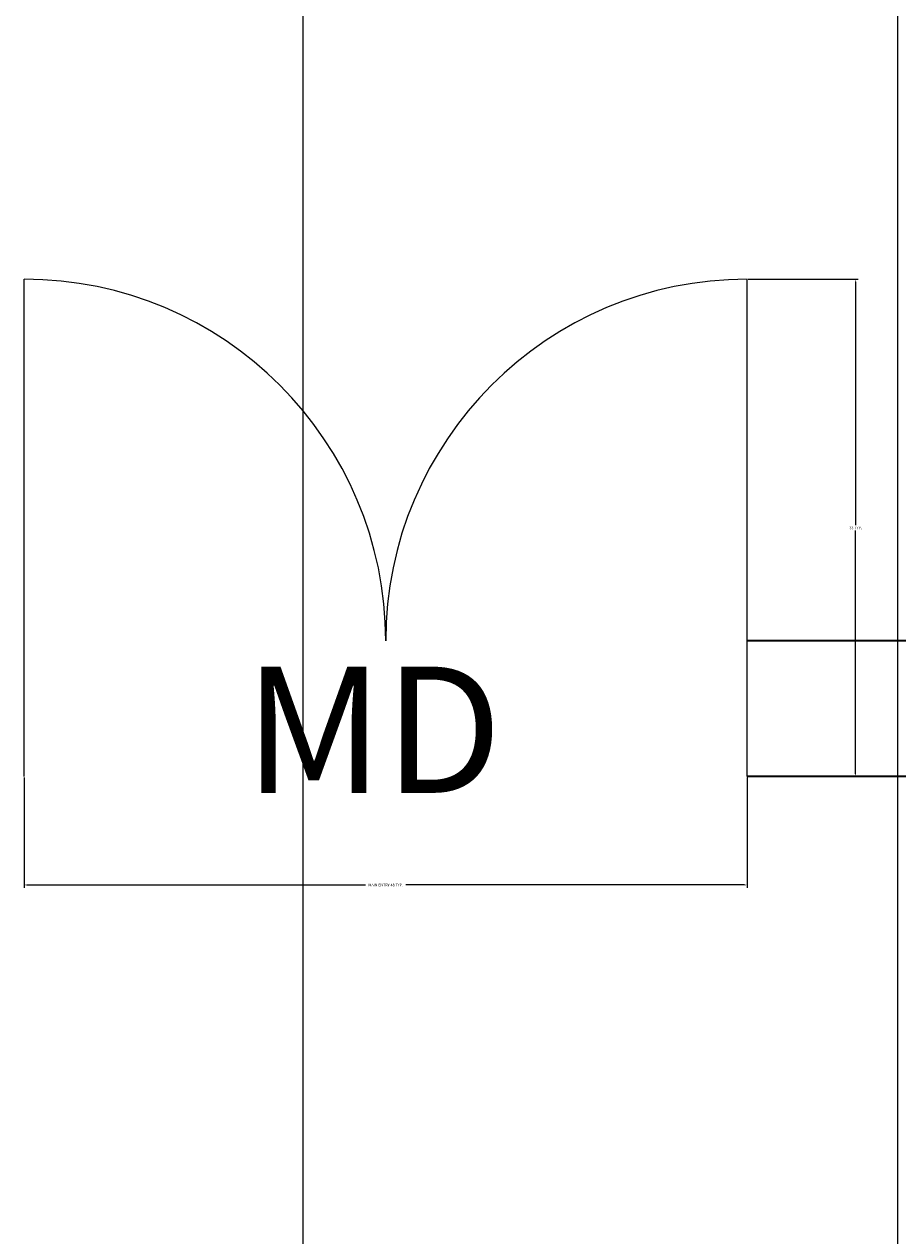
# Model space of a CAD drawing. Units: feet. Extents: x 1654 to 2985, y 1348 to 2230.
# Tile 44 of 53: x 2655 to 2713, y 1712 to 1792. Entities that reach past the tile are written whole.
import ezdxf

# ---------------------------------------------------------------- set-up
doc = ezdxf.new("R2010")
doc.units = ezdxf.units.FT
for name, color, linetype, lineweight in [('A-ANNO-DIMS', 2, 'Continuous', 18), ('A-ANNO-TEXT', 7, 'Continuous', 18), ('A-DOOR', 3, 'Continuous', 18), ('A-WALL', 7, 'Continuous', 35)]:
    doc.layers.add(name, color=color, linetype=linetype, lineweight=lineweight)
doc.styles.get("Standard").update_dxf_attribs({"font": 'arial.ttf'})
doc.dimstyles.get("Standard").update_dxf_attribs({"dimtxt": 0.18, "dimasz": 0.18, "dimexe": 0.18, "dimexo": 0.0625, "dimgap": 0.09, "dimtad": 0, "dimtih": 1, "dimtoh": 1, "dimdec": 4, "dimzin": 0, "dimdsep": 46, "dimtxsty": 'Standard', "dimcen": 0.09, "dimadec": 0, "dimazin": 0, "dimtfac": 1, "dimtdec": 4, "dimtofl": 0, "dimtmove": 0, "dimatfit": 3, "dimfxl": 1, "dimtolj": 1, "dimtzin": 0, "dimarcsym": 0})

# ---------------------------------------------------------------- blocks, each defined once
blk = doc.blocks.new('DOOR-ENTRY-PAIR')
for p, q in [((0, -9), (0, 24)), ((48, -9), (48, 24))]:
    blk.add_line(p, q)
for centre, start, end in [((0, 0), 0, 90), ((48, 0), 90, 180)]:
    blk.add_arc(centre, 24, start, end)
blk = doc.blocks.new('*D32')
at = {"layer": 'A-ANNO-DIMS', "color": 0, "lineweight": -2, "transparency": 16777216}
for p, q in [((2654.706, 1742.192), (2654.706, 1734.875)), ((2702.706, 1742.192), (2702.706, 1734.875)), ((2654.886, 1735.055), (2677.372, 1735.055)), ((2702.526, 1735.055), (2680.04, 1735.055))]:
    blk.add_line(p, q, dxfattribs=at)
at = {"layer": 'A-ANNO-DIMS', "color": 0, "transparency": 16777216}
for points in [[(2654.886, 1735.085), (2654.886, 1735.025), (2654.706, 1735.055)], [(2702.526, 1735.085), (2702.526, 1735.025), (2702.706, 1735.055)]]:
    blk.add_solid(points, dxfattribs=at)
at = {"layer": 'Defpoints', "color": 0, "transparency": 16777216}
for p in [(2654.706, 1742.255), (2702.706, 1742.255), (2702.706, 1735.055)]:
    blk.add_point(p, dxfattribs=at)
at = {"layer": 'A-ANNO-DIMS', "color": 0, "transparency": 16777216, "insert": (2678.706, 1735.055), "char_height": 0.18, "attachment_point": 5}
blk.add_mtext('\\A1;MAIN ENTRY 48 TYP.', dxfattribs=at)
blk = doc.blocks.new('*D33')
at = {"layer": 'A-ANNO-DIMS', "color": 0, "lineweight": -2, "transparency": 16777216}
for p, q in [((2702.768, 1775.255), (2710.086, 1775.255)), ((2709.906, 1775.075), (2709.906, 1758.937)), ((2709.906, 1742.435), (2709.906, 1758.573)), ((2702.768, 1742.255), (2710.086, 1742.255))]:
    blk.add_line(p, q, dxfattribs=at)
at = {"layer": 'A-ANNO-DIMS', "color": 0, "transparency": 16777216}
for points in [[(2709.876, 1775.075), (2709.936, 1775.075), (2709.906, 1775.255)], [(2709.876, 1742.435), (2709.936, 1742.435), (2709.906, 1742.255)]]:
    blk.add_solid(points, dxfattribs=at)
at = {"layer": 'Defpoints', "color": 0, "transparency": 16777216}
for p in [(2702.706, 1775.255), (2709.906, 1775.255), (2702.706, 1742.255)]:
    blk.add_point(p, dxfattribs=at)
at = {"layer": 'A-ANNO-DIMS', "color": 0, "transparency": 16777216, "insert": (2709.906, 1758.755), "char_height": 0.18, "attachment_point": 5}
blk.add_mtext('\\A1;33 TYP.', dxfattribs=at)
blk = doc.blocks.new('*D82')
at = {"layer": 'A-ANNO-DIMS', "color": 0, "lineweight": -2, "transparency": 16777216}
for p, q in [((2652.706, 2039.192), (2652.706, 1490.625)), ((2784.706, 2039.192), (2784.706, 1490.625)), ((2652.886, 1490.805), (2718.426, 1490.805)), ((2784.526, 1490.805), (2718.985, 1490.805))]:
    blk.add_line(p, q, dxfattribs=at)
at = {"layer": 'A-ANNO-DIMS', "color": 0, "transparency": 16777216}
for points in [[(2652.886, 1490.835), (2652.886, 1490.775), (2652.706, 1490.805)], [(2784.526, 1490.835), (2784.526, 1490.775), (2784.706, 1490.805)]]:
    blk.add_solid(points, dxfattribs=at)
at = {"layer": 'Defpoints', "color": 0, "transparency": 16777216}
for p in [(2652.706, 2039.255), (2784.706, 2039.255), (2784.706, 1490.805)]:
    blk.add_point(p, dxfattribs=at)
at = {"layer": 'A-ANNO-DIMS', "color": 0, "transparency": 16777216, "insert": (2718.706, 1490.805), "char_height": 0.18, "attachment_point": 5}
blk.add_mtext('\\A1;132', dxfattribs=at)
blk = doc.blocks.new('*D84')
at = {"layer": 'A-ANNO-DIMS', "color": 0, "lineweight": -2, "transparency": 16777216}
for p, q in [((2625.235, 1565.317), (2625.235, 2149.885)), ((2625.415, 2149.705), (2649.013, 2149.705)), ((2673.055, 2149.705), (2649.458, 2149.705)), ((2673.235, 1565.317), (2673.235, 2149.885))]:
    blk.add_line(p, q, dxfattribs=at)
at = {"layer": 'A-ANNO-DIMS', "color": 0, "transparency": 16777216}
for points in [[(2625.415, 2149.735), (2625.415, 2149.675), (2625.235, 2149.705)], [(2673.055, 2149.735), (2673.055, 2149.675), (2673.235, 2149.705)]]:
    blk.add_solid(points, dxfattribs=at)
at = {"layer": 'Defpoints', "color": 0, "transparency": 16777216}
for p in [(2673.235, 2149.705), (2625.235, 1565.255), (2673.235, 1565.255)]:
    blk.add_point(p, dxfattribs=at)
at = {"layer": 'A-ANNO-DIMS', "color": 0, "transparency": 16777216, "insert": (2649.235, 2149.705), "char_height": 0.18, "attachment_point": 5}
blk.add_mtext('\\A1;48', dxfattribs=at)
blk = doc.blocks.new('*D85')
at = {"layer": 'A-ANNO-DIMS', "color": 0, "lineweight": -2, "transparency": 16777216}
for p, q in [((2673.235, 1565.317), (2673.235, 2149.885)), ((2673.415, 2149.705), (2692.577, 2149.705)), ((2712.526, 2149.705), (2693.364, 2149.705)), ((2712.706, 1565.317), (2712.706, 2149.885))]:
    blk.add_line(p, q, dxfattribs=at)
at = {"layer": 'A-ANNO-DIMS', "color": 0, "transparency": 16777216}
for points in [[(2673.415, 2149.735), (2673.415, 2149.675), (2673.235, 2149.705)], [(2712.526, 2149.735), (2712.526, 2149.675), (2712.706, 2149.705)]]:
    blk.add_solid(points, dxfattribs=at)
at = {"layer": 'Defpoints', "color": 0, "transparency": 16777216}
for p in [(2712.706, 2149.705), (2673.235, 1565.255), (2712.706, 1565.255)]:
    blk.add_point(p, dxfattribs=at)
at = {"layer": 'A-ANNO-DIMS', "color": 0, "transparency": 16777216, "insert": (2692.971, 2149.705), "char_height": 0.18, "attachment_point": 5}
blk.add_mtext('\\A1;39.47', dxfattribs=at)

msp = doc.modelspace()

# ---------------------------------------------------------------- linework, layer by layer
at = {"layer": 'A-WALL'}
for p, q in [((2784.7058, 1751.2549), (2702.7058, 1751.2549)), ((2784.7058, 1742.2549), (2702.7058, 1742.2549))]:
    msp.add_line(p, q, dxfattribs=at)

# ---------------------------------------------------------------- block references
at = {"layer": 'A-DOOR'}
msp.add_blockref('DOOR-ENTRY-PAIR', (2654.7058, 1751.2549), dxfattribs=at)

# ---------------------------------------------------------------- texts
at = {"layer": 'A-ANNO-TEXT'}
msp.add_text('MD', height=8.38114, dxfattribs=at).set_placement((2669.2983, 1741.1636))

# ---------------------------------------------------------------- dimensions: what is measured, and where the dimension line sits
at = {"layer": 'A-ANNO-DIMS'}
for base, p1, p2, override, picture, middle in [((2673.2353, 2149.7049), (2625.2353, 1565.2549), (2673.2353, 1565.2549), {"dimdec": 0, "dimlfac": 1, "dimrnd": 0, "dimzin": 0, "dimdsep": 46, "dimlunit": 2}, '*D84', (2649.2353, 2149.7049)), ((2712.7058, 2149.7049), (2673.2353, 1565.2549), (2712.7058, 1565.2549), {"dimdec": 2, "dimlfac": 1, "dimrnd": 0, "dimzin": 0, "dimdsep": 46, "dimlunit": 2}, '*D85', (2692.9706, 2149.7049)), ((2784.7058, 1490.8049), (2652.7058, 2039.2549), (2784.7058, 2039.2549), {"dimdec": 0, "dimlfac": 1, "dimrnd": 0, "dimzin": 0, "dimdsep": 46, "dimlunit": 2}, '*D82', (2718.7058, 1490.8049))]:
    dim = msp.add_linear_dim(base=base, p1=p1, p2=p2, dimstyle='Standard', override=override, dxfattribs=at)
    dim.commit()
    dim.dimension.update_dxf_attribs({"geometry": picture, "text_midpoint": middle})
dim = msp.add_linear_dim(base=(2709.9058, 1775.2549), p1=(2702.7058, 1742.2549), p2=(2702.7058, 1775.2549), angle=90, text='<> TYP.', dimstyle='Standard', override={"dimdec": 0, "dimlfac": 1, "dimrnd": 0, "dimzin": 0, "dimdsep": 46, "dimlunit": 2}, dxfattribs=at)
dim.commit()
dim.dimension.update_dxf_attribs({"geometry": '*D33', "text_midpoint": (2709.9058, 1758.7549)})
dim = msp.add_linear_dim(base=(2702.7058, 1735.0549), p1=(2654.7058, 1742.2549), p2=(2702.7058, 1742.2549), text='MAIN ENTRY <> TYP.', dimstyle='Standard', override={"dimdec": 0, "dimlfac": 1, "dimrnd": 0, "dimzin": 0, "dimdsep": 46, "dimlunit": 2}, dxfattribs=at)
dim.commit()
dim.dimension.update_dxf_attribs({"geometry": '*D32', "text_midpoint": (2678.7058, 1735.0549)})

doc.saveas('drawing.dxf')
